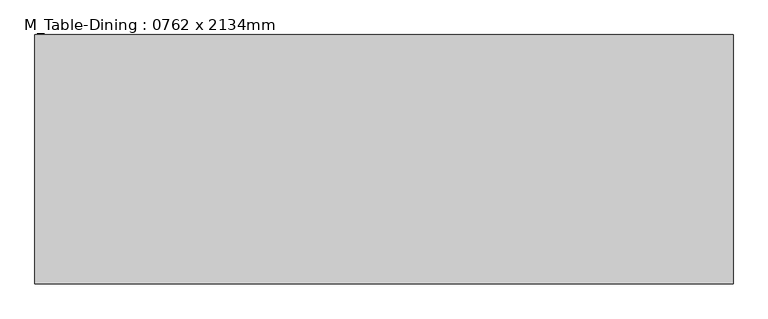
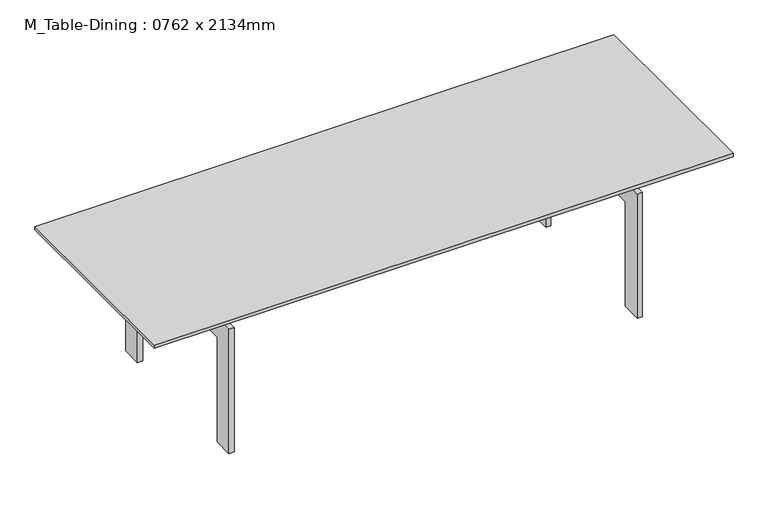
"""IFC4 building model written with IfcOpenShell, lengths in millimetres: furniture geometry, M_Table-Dining : 0762 x 2134mm."""

from ifc_helpers import new_model, si_unit, frame, origin, place, context, project, spatial, polyline, outline, extrude, source, transform, mapped, element, save


def m_table_dining_0762_x_2134mm_32ec0f49(model_context):
    return source(origin(), model_context, "Body", "SweptSolid", [
        extrude(outline(polyline([(1085.2657667, 476.2110778), (1085.2657667, -285.7889222), (-1048.7342333, -285.7889222), (-1048.7342333, 476.2110778), (1085.2657667, 476.2110778)])), frame((0.0, 0.0, 547.3), z_axis=(0.0, 0.0, 1.0), x_axis=(1.0, 0.0, 0.0)), (0.0, 0.0, 1.0), 12.7),
        extrude(outline(polyline([(425.4110778, 483.8), (425.4110778, 0.0), (349.2110778, 0.0), (349.2110778, 407.6), (-158.7889222, 407.6), (-158.7889222, 0.0), (-234.9889222, 0.0), (-234.9889222, 483.8), (425.4110778, 483.8)])), frame((-743.9342333, 0.0, 0.0), z_axis=(1.0, 0.0, 0.0), x_axis=(0.0, 1.0, 0.0)), (0.0, 0.0, 1.0), 19.05),
        extrude(outline(polyline([(425.4110778, 0.0), (349.2110778, 0.0), (349.2110778, 407.6), (-158.7889222, 407.6), (-158.7889222, 0.0), (-234.9889222, 0.0), (-234.9889222, 483.8), (425.4110778, 483.8), (425.4110778, 0.0)])), frame((761.4157667, 0.0, 0.0), z_axis=(1.0, 0.0, 0.0), x_axis=(0.0, 1.0, 0.0)), (0.0, 0.0, 1.0), 19.05),
        extrude(outline(polyline([(983.6657667, 297.7823857), (983.6657667, 272.3823857), (-947.1342333, 272.3823857), (-947.1342333, 297.7823857), (983.6657667, 297.7823857)])), frame((0.0, 0.0, 483.8), z_axis=(0.0, 0.0, 1.0), x_axis=(1.0, 0.0, 0.0)), (0.0, 0.0, 1.0), 63.5),
        extrude(outline(polyline([(983.6657667, -82.5889222), (983.6657667, -107.9889222), (-947.1342333, -107.9889222), (-947.1342333, -82.5889222), (983.6657667, -82.5889222)])), frame((0.0, 0.0, 483.8), z_axis=(0.0, 0.0, 1.0), x_axis=(1.0, 0.0, 0.0)), (0.0, 0.0, 1.0), 63.5),
    ])


if __name__ == "__main__":
    model = new_model("IFC4")
    model_context = context("Model", 3, world=origin())
    ifc_project = project(units=[si_unit("LENGTHUNIT", "METRE", prefix="MILLI")], contexts=[model_context])
    site = spatial("IfcSite", under=ifc_project)
    building = spatial("IfcBuilding", under=site)
    placement = place(None, origin())
    m_table_dining_0762_x_2134mm_shape = m_table_dining_0762_x_2134mm_32ec0f49(model_context)
    element("IfcFurniture", 1, ObjectType="M_Table-Dining : 0762 x 2134mm", at=placement, inside=building, context=model_context, shape_type="MappedRepresentation", body=[
        mapped(m_table_dining_0762_x_2134mm_shape, transform((0.0, 0.0, 0.0), x_axis=(1.0, 0.0, 0.0), y_axis=(0.0, 1.0, 0.0), z_axis=(0.0, 0.0, 1.0))),
    ])
    save(model, "model.ifc")

# Revit data of these elements
# Type "M_Table-Dining : 0762 x 2134mm"
#   Height = 560 mm
#   Length = 2134 mm
#   Width = 762 mm
#   Base Material = Steel, Chrome Plated
#   Top Material = Glass - Clear, Grey
#   Default Elevation = 0
# Element 1 (IfcFurniture, "M_Table-Dining : 0762 x 2134mm")
#   Materials on its faces: "Steel, Chrome Plated", "Glass - Clear, Grey"
# Materials
#   "Steel, Chrome Plated": class "Metal", colour RGB 17 17 17, transparency 0, Description = "Chromiuim plated steel", Cost = 0
#   "Glass - Clear, Grey": class "Glass", colour RGB 252 255 255, transparency 0.64
